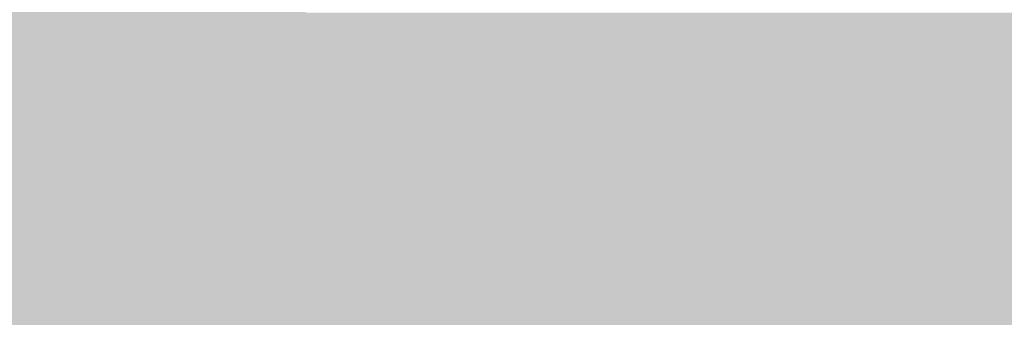
# Model space of a CAD drawing. Units: feet. Extents: x 3168 to 4724, y 827 to 1477.
# Tile 124 of 256: x 3298.685 to 3300.858, y 1098.344 to 1099.001. Entities that reach past the tile are written whole.
import ezdxf

# ---------------------------------------------------------------- set-up
doc = ezdxf.new("R2010")
doc.units = ezdxf.units.FT
doc.layers.add('A-ELEV', color=7, linetype='Continuous', lineweight=35)
doc.layers.add('A-ELEV-PATT', color=8, linetype='Continuous', lineweight=13)

msp = doc.modelspace()

# ---------------------------------------------------------------- hatches: boundary and pattern name
at = {"layer": 'A-ELEV-PATT'}
h = msp.add_hatch(color=256, dxfattribs=at)
h.dxf.hatch_style = 1
edge = h.paths.add_edge_path()
edge.add_ellipse((3552.9058, 979.2201), major_axis=(36.7449, 0), ratio=0.4848485, start_angle=0, end_angle=360)
edge = h.paths.add_edge_path()
edge.add_ellipse((3559.8916, 929.2523), major_axis=(36.7449, 0), ratio=0.4848485, start_angle=0, end_angle=360)
edge = h.paths.add_edge_path()
edge.add_line((3299.3168, 1198.6061), (3479.9167, 1198.6061))
edge.add_line((3479.9167, 1198.6061), (3479.9167, 1209.8686))
edge.add_spline(control_points=[(3479.9167, 1209.8686), (3464.3012, 1209.8686), (3448.6856, 1209.8686), (3410.9491, 1209.8686), (3388.8282, 1209.8686), (3355.6469, 1209.8686), (3344.5864, 1209.8686), (3327.9957, 1209.8686), (3322.4655, 1209.8686), (3314.1702, 1209.8686), (3311.4051, 1209.8686), (3307.2574, 1209.8686), (3305.8748, 1209.8686), (3303.801, 1209.8686), (3303.1097, 1209.8686), (3302.0728, 1209.8686), (3301.7272, 1209.8686), (3301.2087, 1209.8686), (3301.0359, 1209.8686), (3300.7767, 1209.8686), (3300.6903, 1209.8686), (3300.5606, 1209.8686), (3300.5174, 1209.8686), (3300.4526, 1209.8686), (3300.431, 1209.8686), (3300.3986, 1209.8686), (3300.3878, 1209.8686), (3300.3662, 1209.8686), (3300.3457, 1209.8686), (3300.3455, 1209.8686), (3300.3455, 1209.8686), (3300.3433, 1209.8686), (3300.3411, 1209.8686), (3300.3379, 1209.8686), (3300.3368, 1209.8686), (3300.3339, 1209.8686), (3300.3321, 1209.8686), (3300.3255, 1209.8686), (3300.3207, 1209.8686), (3300.3109, 1209.8686), (3300.306, 1209.8686), (3300.2905, 1209.8686), (3300.28, 1209.8686), (3300.2324, 1209.8688), (3300.1953, 1209.869), (3299.9511, 1209.8706), (3299.7448, 1209.8743), (3299.4368, 1209.8833), (3299.3344, 1209.8868), (3299.1811, 1209.8929), (3299.13, 1209.8951), (3298.6522, 1209.9168), (3298.2295, 1209.9457), (3297.6016, 1210.0024), (3297.3934, 1210.0235), (3297.0827, 1210.0583), (3296.9793, 1210.0705), (3296.293, 1210.1549), (3295.7181, 1210.2434), (3294.8687, 1210.3989), (3294.5877, 1210.4545), (3294.1693, 1210.5433), (3294.0304, 1210.5739), (3291.7071, 1211.1012), (3289.6536, 1211.8134), (3285.7763, 1213.564), (3283.9514, 1214.6035), (3280.5122, 1216.9801), (3278.8972, 1218.3176), (3276.3799, 1220.8295), (3275.416, 1221.9177), (3274.0393, 1223.7077), (3273.581, 1224.3495), (3273.1432, 1225.0163)], knot_values=[39.119033, 39.119033, 39.119033, 39.119033, 39.286353, 39.286353, 39.523379, 39.523379, 39.641892, 39.641892, 39.701148, 39.701148, 39.730777, 39.730777, 39.745591, 39.745591, 39.752998, 39.752998, 39.756701, 39.756701, 39.758553, 39.758553, 39.759479, 39.759479, 39.759942, 39.759942, 39.760173, 39.760173, 39.760289, 39.760289, 39.760405, 39.760405, 39.760463, 39.760463, 39.763389, 39.763389, 39.764851, 39.764851, 39.767304, 39.767304, 39.773825, 39.773825, 39.78057, 39.78057, 39.79477, 39.79477, 39.845194, 39.845194, 40.126715, 40.126715, 40.267476, 40.267476, 40.337856, 40.337856, 40.927023, 40.927023, 41.221606, 41.221606, 41.368898, 41.368898, 42.202622, 42.202622, 42.619485, 42.619485, 42.827916, 42.827916, 46.118323, 46.118323, 49.408731, 49.408731, 52.699139, 52.699139, 54.927489, 54.927489, 56.104228, 56.104228, 56.104228, 56.104228], weights=[1, 1, 1, 1, 1, 1, 1, 1, 1, 1, 1, 1, 1, 1, 1, 1, 1, 1, 1, 1, 1, 1, 1, 1, 1, 1, 1, 1, 1, 1, 1, 1, 1, 1, 1, 1, 1, 1, 1, 1, 1, 1, 1, 1, 1, 1, 1, 1, 1, 1, 1, 1, 1, 1, 1, 1, 1, 1, 1, 1, 1, 1, 1, 1, 1, 1, 1, 1, 1, 1, 1, 1, 1, 1], degree=3, periodic=0)
edge.add_line((3273.1432, 1225.0163), (3273.1432, 1099.0163))
edge.add_line((3273.1432, 1099.0163), (3299.3168, 1099.0163))
edge.add_line((3299.3168, 1099.0163), (3299.3168, 1198.6061))
edge = h.paths.add_edge_path()
edge.add_line((3304.7584, 1324.1581), (3479.9167, 1324.1581))
edge.add_line((3479.9167, 1324.1581), (3479.9167, 1335.7146))
edge.add_line((3479.9167, 1335.7146), (3269.1616, 1335.7146))
edge.add_spline(control_points=[(3269.1616, 1335.7146), (3264.0242, 1335.7146), (3258.3641, 1328.9582), (3259.2643, 1323.9003)], knot_values=[0, 0, 0, 0, 15.412191, 15.412191, 15.412191, 15.412191], degree=3, periodic=0)
edge.add_line((3259.2643, 1323.9003), (3265.5168, 1288.7691))
edge.add_line((3265.5168, 1288.7691), (3275.2651, 1261.5456))
edge.add_line((3275.2651, 1261.5456), (3304.7584, 1261.5456))
edge.add_line((3304.7584, 1261.5456), (3304.7584, 1324.1581))
h = msp.add_hatch(color=256, dxfattribs=at)
h.dxf.hatch_style = 1
h.paths.add_polyline_path([(3384.5252, 1099.0163), (3335.0292, 1099.0163), (3299.3168, 1099.0163), (3273.1432, 1099.0163), (3217.5654, 1099.0163), (3168.0693, 827.1163), (3335.0292, 827.1163)])

# ---------------------------------------------------------------- linework, layer by layer
at = {"layer": 'A-ELEV'}
msp.add_open_spline([(3808.5202, 1099.0163), (3808.5202, 1141.4132), (3808.5202, 1183.8102), (3808.5202, 1226.6353), (3808.5202, 1227.0636), (3808.5202, 1227.4918), (3811.4919, 1248.9947), (3814.4635, 1270.4975), (3817.4652, 1292.2176), (3817.4952, 1292.4348), (3817.5253, 1292.652), (3817.5728, 1310.1067), (3817.6203, 1327.5615), (3817.6679, 1345.0163), (3817.6679, 1345.458), (3817.6679, 1345.8996), (3817.6679, 1346.456), (3817.6679, 1346.5708), (3817.6679, 1346.7529), (3817.6679, 1346.8201), (3817.6679, 1346.9349), (3817.6679, 1346.9823), (3817.6679, 1347.0386), (3817.6679, 1347.0474), (3817.6679, 1347.0737), (3817.6679, 1347.0593), (3817.6679, 1347.0615), (3817.6679, 1347.0627), (3817.6679, 1347.066), (3817.6679, 1347.0683), (3817.6679, 1347.075), (3817.6679, 1347.0795), (3817.6678, 1347.0929), (3817.6678, 1347.1019), (3817.6678, 1347.1288), (3817.6677, 1347.1467), (3817.6674, 1347.2004), (3817.6672, 1347.2362), (3817.6661, 1347.3434), (3817.665, 1347.4147), (3817.6608, 1347.6281), (3817.6566, 1347.7697), (3817.64, 1348.1925), (3817.6235, 1348.4716), (3817.5591, 1349.3001), (3817.4961, 1349.8406), (3817.2554, 1351.4242), (3817.0263, 1352.4288), (3816.3069, 1354.8889), (3815.7437, 1356.2687), (3814.464, 1358.8192), (3813.7464, 1359.991), (3812.1958, 1362.1723), (3811.3622, 1363.1821), (3809.5888, 1365.069), (3808.6488, 1365.9461), (3806.6543, 1367.5796), (3805.5997, 1368.3362), (3803.3529, 1369.7223), (3802.1605, 1370.3524), (3799.6008, 1371.4536), (3798.2327, 1371.9255), (3795.2801, 1372.6346), (3793.6931, 1372.8721), (3791.8694, 1372.9265), (3791.7409, 1372.9292), (3791.3534, 1372.9341), (3791.0927, 1372.9329), (3790.3041, 1372.9151), (3789.7695, 1372.8842), (3789.2092, 1372.8302), (3789.1906, 1372.8284), (3789.1349, 1372.8229), (3789.0977, 1372.8191), (3789.0484, 1372.814), (3789.0364, 1372.8127), (3789.0003, 1372.8089), (3788.9761, 1372.8063), (3788.9494, 1372.8034), (3788.9468, 1372.8031), (3788.9426, 1372.8027), (3788.941, 1372.8025), (3788.9386, 1372.8022), (3788.9378, 1372.8021), (3788.9354, 1372.8019), (3788.8675, 1372.7944), (3788.7569, 1372.7822), (3788.7015, 1372.7761), (3788.5355, 1372.7579), (3788.4249, 1372.7457), (3788.0929, 1372.7092), (3787.8715, 1372.6848), (3787.2075, 1372.6118), (3786.7648, 1372.5631), (3785.4368, 1372.417), (3784.5515, 1372.3196), (3781.8954, 1372.0274), (3780.1247, 1371.8327), (3774.8126, 1371.2483), (3771.2713, 1370.8587), (3760.6471, 1369.69), (3753.5643, 1368.9109), (3732.316, 1366.5735), (3718.1504, 1365.0152), (3694.0068, 1362.3593), (3684.0287, 1361.2617), (3674.0506, 1360.1641), (3664.6007, 1360.1641), (3655.1508, 1360.1641), (3626.8011, 1360.1641), (3607.9013, 1360.1641), (3551.2019, 1360.1641), (3513.4023, 1360.1641), (3467.7252, 1360.1641), (3459.8476, 1360.1641), (3436.2149, 1360.1641), (3420.4597, 1360.1641), (3373.1943, 1360.1641), (3341.6839, 1360.1641), (3302.8482, 1360.1641), (3295.5227, 1360.1641), (3286.0383, 1360.1641), (3283.8794, 1360.1641), (3277.4026, 1360.1641), (3273.0848, 1360.1641), (3267.7329, 1360.1641), (3266.6988, 1360.1641), (3263.5965, 1360.1641), (3261.5284, 1360.1641), (3259.2369, 1360.1641), (3259.0137, 1360.1641), (3258.344, 1360.1641), (3257.8975, 1360.1641), (3257.431, 1360.1641), (3257.411, 1360.1641), (3257.3706, 1360.1641), (3257.3755, 1360.1641), (3257.3746, 1360.1641), (3257.3739, 1360.1641), (3257.372, 1360.1641), (3257.3706, 1360.1641), (3257.3667, 1360.1641), (3257.364, 1360.1641), (3257.3561, 1360.1641), (3257.3508, 1360.164), (3257.335, 1360.164), (3257.3244, 1360.164), (3257.2928, 1360.1639), (3257.2717, 1360.1638), (3257.2084, 1360.1634), (3257.1663, 1360.163), (3257.0402, 1360.1614), (3256.9563, 1360.1598), (3256.7055, 1360.1534), (3256.5392, 1360.147), (3256.0436, 1360.1219), (3255.7173, 1360.0971), (3254.7524, 1360.0005), (3254.128, 1359.9065), (3252.1801, 1359.5253), (3250.9416, 1359.144), (3248.6702, 1358.2433), (3247.6357, 1357.7238), (3245.7326, 1356.6035), (3244.8634, 1356.0021), (3243.2531, 1354.7429), (3242.512, 1354.0847), (3240.7511, 1352.3448), (3239.801, 1351.2296), (3238.0878, 1348.8724), (3237.3247, 1347.6304), (3235.9825, 1344.9716), (3235.4022, 1343.5549), (3234.5911, 1340.8155), (3234.3109, 1339.5435), (3233.9765, 1336.8026), (3233.9221, 1335.3309), (3234.1489, 1332.5913), (3234.3495, 1331.3672), (3234.7199, 1329.9994), (3234.7524, 1329.8834), (3234.8536, 1329.5348), (3234.9259, 1329.3017), (3235.0248, 1329.0026), (3235.0469, 1328.9369), (3235.0776, 1328.8472), (3235.0859, 1328.8232), (3235.1109, 1328.7511), (3235.1278, 1328.703), (3235.148, 1328.6462), (3235.1511, 1328.6376), (3235.1561, 1328.6235), (3235.1581, 1328.618), (3235.1602, 1328.612), (3235.1656, 1328.5969), (3235.1801, 1328.5565), (3235.1903, 1328.5281), (3235.2208, 1328.4429), (3235.2411, 1328.3862), (3235.3021, 1328.2159), (3235.3427, 1328.1023), (3235.4647, 1327.7617), (3235.546, 1327.5346), (3235.79, 1326.8534), (3235.9526, 1326.3992), (3236.4405, 1325.0367), (3236.7657, 1324.1284), (3237.7415, 1321.4034), (3238.392, 1319.5868), (3240.3435, 1314.1369), (3241.6445, 1310.5036), (3245.5476, 1299.6037), (3248.1496, 1292.3371), (3255.9557, 1270.5374), (3261.1598, 1256.0042), (3267.3876, 1238.612), (3268.4114, 1235.7529), (3269.5104, 1232.6839), (3269.5856, 1232.4739), (3269.7066, 1232.1359), (3269.7524, 1232.0079), (3269.8273, 1231.7987), (3269.8564, 1231.7176), (3269.9063, 1231.5781), (3269.9272, 1231.5198), (3269.9725, 1231.3934), (3269.9968, 1231.3254), (3270.0265, 1231.2425), (3270.0318, 1231.2277), (3270.0403, 1231.204), (3270.0392, 1231.207), (3270.0394, 1231.2066), (3270.0394, 1231.2064), (3270.0396, 1231.2058), (3270.0398, 1231.2055), (3270.0402, 1231.2043), (3270.0404, 1231.2036), (3270.0413, 1231.2013), (3270.0418, 1231.1998), (3270.0434, 1231.1953), (3270.0445, 1231.1922), (3270.0478, 1231.1832), (3270.0499, 1231.1771), (3270.0564, 1231.159), (3270.0608, 1231.147), (3270.0739, 1231.1108), (3270.0826, 1231.0867), (3270.1089, 1231.0144), (3270.1266, 1230.9663), (3270.1799, 1230.8225), (3270.2159, 1230.7269), (3270.3253, 1230.4415), (3270.4, 1230.2528), (3270.6292, 1229.6914), (3270.7889, 1229.3235), (3271.2865, 1228.2383), (3271.6431, 1227.5398), (3272.7759, 1225.5153), (3273.6142, 1224.2605), (3275.416, 1221.9177), (3276.3799, 1220.8295), (3278.8972, 1218.3176), (3280.5122, 1216.9801), (3283.9514, 1214.6035), (3285.7763, 1213.564), (3289.6536, 1211.8134), (3291.7071, 1211.1012), (3294.0304, 1210.5739), (3294.1693, 1210.5433), (3294.5877, 1210.4545), (3294.8687, 1210.3989), (3295.7181, 1210.2434), (3296.293, 1210.1549), (3296.9793, 1210.0705), (3297.0827, 1210.0583), (3297.3934, 1210.0235), (3297.6016, 1210.0024), (3298.2295, 1209.9457), (3298.6522, 1209.9168), (3299.13, 1209.8951), (3299.1811, 1209.8929), (3299.3344, 1209.8868), (3299.4368, 1209.8833), (3299.7448, 1209.8743), (3299.9511, 1209.8706), (3300.1953, 1209.869), (3300.2324, 1209.8688), (3300.28, 1209.8686), (3300.2905, 1209.8686), (3300.306, 1209.8686), (3300.3109, 1209.8686), (3300.3207, 1209.8686), (3300.3255, 1209.8686), (3300.3321, 1209.8686), (3300.3339, 1209.8686), (3300.3368, 1209.8686), (3300.3379, 1209.8686), (3300.3411, 1209.8686), (3300.3433, 1209.8686), (3300.3455, 1209.8686), (3300.3455, 1209.8686), (3300.3457, 1209.8686), (3300.3662, 1209.8686), (3300.3878, 1209.8686), (3300.3986, 1209.8686), (3300.431, 1209.8686), (3300.4526, 1209.8686), (3300.5174, 1209.8686), (3300.5606, 1209.8686), (3300.6903, 1209.8686), (3300.7767, 1209.8686), (3301.0359, 1209.8686), (3301.2087, 1209.8686), (3301.7272, 1209.8686), (3302.0728, 1209.8686), (3303.1097, 1209.8686), (3303.801, 1209.8686), (3305.8748, 1209.8686), (3307.2574, 1209.8686), (3311.4051, 1209.8686), (3314.1702, 1209.8686), (3322.4655, 1209.8686), (3327.9957, 1209.8686), (3344.5864, 1209.8686), (3355.6469, 1209.8686), (3388.8282, 1209.8686), (3410.9491, 1209.8686), (3477.3119, 1209.8686), (3521.5537, 1209.8686), (3566.8362, 1209.8686), (3567.8769, 1209.8686), (3570.999, 1209.8686), (3573.0804, 1209.8686), (3575.7814, 1209.8686), (3576.4009, 1209.8686), (3577.2958, 1209.8686), (3577.5712, 1209.8686), (3578.3971, 1209.8686), (3578.9478, 1209.8686), (3579.7565, 1209.8686), (3580.0145, 1209.8686), (3580.3427, 1209.8686), (3580.3269, 1209.8686), (3580.3272, 1209.8686), (3580.3273, 1209.8686), (3580.3278, 1209.8686), (3580.3281, 1209.8686), (3580.329, 1209.8686), (3580.3296, 1209.8686), (3580.3314, 1209.8686), (3580.3327, 1209.8686), (3580.3363, 1209.8686), (3580.3388, 1209.8686), (3580.3461, 1209.8686), (3580.351, 1209.8686), (3580.3657, 1209.8685), (3580.3754, 1209.8685), (3580.4048, 1209.8684), (3580.4244, 1209.8684), (3580.4832, 1209.8681), (3580.5224, 1209.8678), (3580.6404, 1209.8666), (3580.7192, 1209.8655), (3580.9563, 1209.8608), (3581.1152, 1209.8561), (3581.5942, 1209.8372), (3581.9164, 1209.8183), (3582.8899, 1209.7424), (3583.548, 1209.6662), (3585.5318, 1209.3606), (3586.8672, 1209.0539), (3589.4715, 1208.2525), (3590.7402, 1207.7579), (3591.9955, 1207.1588), (3592.0578, 1207.1287), (3592.2442, 1207.038), (3592.3677, 1206.9766), (3592.7353, 1206.7904), (3592.9768, 1206.6631), (3593.2445, 1206.5164), (3593.2747, 1206.4998), (3593.3651, 1206.4498), (3593.4251, 1206.4163), (3593.6043, 1206.3153), (3593.7227, 1206.2472), (3593.8572, 1206.1684), (3593.8744, 1206.1583), (3593.9257, 1206.128), (3593.9599, 1206.1078), (3594.0621, 1206.0469), (3594.1298, 1206.0061), (3594.2084, 1205.9582), (3594.2197, 1205.9513), (3594.2534, 1205.9307), (3594.2758, 1205.9169), (3594.343, 1205.8755), (3594.3876, 1205.8479), (3594.4336, 1205.819), (3594.4353, 1205.818), (3594.4402, 1205.8149), (3594.4435, 1205.8129), (3594.4471, 1205.8106), (3594.4475, 1205.8103), (3594.4487, 1205.8096), (3594.4495, 1205.8091), (3594.4504, 1205.8086), (3594.4505, 1205.8085), (3594.4506, 1205.8084), (3594.4674, 1205.7979), (3594.4933, 1205.7817), (3594.5062, 1205.7736), (3594.545, 1205.7492), (3594.5709, 1205.733), (3594.6485, 1205.6844), (3594.7002, 1205.652), (3594.8554, 1205.5547), (3594.9589, 1205.4898), (3595.2694, 1205.2953), (3595.4763, 1205.1656), (3596.0972, 1204.7765), (3596.5111, 1204.5171), (3597.7528, 1203.7388), (3598.5807, 1203.22), (3601.0642, 1201.6636), (3602.7198, 1200.6259), (3607.6868, 1197.513), (3610.9981, 1195.4377), (3620.932, 1189.2119), (3627.5546, 1185.0614), (3647.4225, 1172.6097), (3660.6678, 1164.3086), (3700.4035, 1139.4053), (3726.894, 1122.8031), (3757.2057, 1103.8061), (3761.027, 1101.4112), (3764.8482, 1099.0163), (3745.3283, 1099.0163), (3725.8083, 1099.0163), (3706.2884, 1099.0163), (3706.2884, 1108.4532), (3706.2884, 1117.8902), (3706.2884, 1127.3271), (3710.7508, 1127.3271), (3715.2131, 1127.3271), (3719.6755, 1127.3271)], degree=3, knots=[0, 0, 0, 0, 0.982037, 0.982037, 0.991957, 0.991957, 0.991957, 1.966522, 1.966522, 1.976367, 1.976367, 1.976367, 2.976367, 2.976367, 2.976367, 3.00169, 3.00169, 3.008272, 3.008272, 3.012129, 3.012129, 3.014851, 3.014851, 3.015353, 3.015353, 3.016359, 3.016359, 3.017365, 3.017365, 3.019376, 3.019376, 3.023398, 3.023398, 3.031442, 3.031442, 3.047531, 3.047531, 3.079708, 3.079708, 3.144063, 3.144063, 3.272772, 3.272772, 3.53019, 3.53019, 4.045026, 4.045026, 5.074698, 5.074698, 6.700878, 6.700878, 8.327058, 8.327058, 9.953238, 9.953238, 11.579418, 11.579418, 13.205598, 13.205598, 14.831778, 14.831778, 16.457958, 16.457958, 18.084138, 18.084138, 18.206872, 18.206872, 18.45234, 18.45234, 18.943275, 18.943275, 18.960093, 18.960093, 18.993729, 18.993729, 19.00461, 19.00461, 19.026374, 19.026374, 19.028737, 19.028737, 19.03018, 19.03018, 19.030897, 19.030897, 19.032332, 19.032332, 19.033766, 19.033766, 19.036636, 19.036636, 19.042374, 19.042374, 19.053851, 19.053851, 19.076805, 19.076805, 19.122714, 19.122714, 19.21453, 19.21453, 19.398163, 19.398163, 19.765429, 19.765429, 20.024128, 20.024128, 20.024128, 20.092031, 20.092031, 20.227836, 20.227836, 20.499446, 20.499446, 20.556051, 20.556051, 20.66926, 20.66926, 20.895678, 20.895678, 20.948316, 20.948316, 20.963829, 20.963829, 20.994855, 20.994855, 21.002285, 21.002285, 21.017146, 21.017146, 21.01875, 21.01875, 21.021959, 21.021959, 21.022102, 21.022102, 21.022249, 21.022249, 21.022708, 21.022708, 21.023627, 21.023627, 21.025464, 21.025464, 21.029138, 21.029138, 21.036486, 21.036486, 21.051183, 21.051183, 21.080575, 21.080575, 21.139361, 21.139361, 21.256932, 21.256932, 21.492073, 21.492073, 21.962356, 21.962356, 23.01002, 23.01002, 24.057684, 24.057684, 25.105348, 25.105348, 26.153011, 26.153011, 27.776787, 27.776787, 29.400562, 29.400562, 31.024337, 31.024337, 32.278801, 32.278801, 33.533265, 33.533265, 34.467568, 34.467568, 34.553971, 34.553971, 34.726776, 34.726776, 34.775309, 34.775309, 34.793079, 34.793079, 34.82862, 34.82862, 34.834979, 34.834979, 34.839039, 34.839039, 34.839411, 34.839411, 34.840285, 34.840285, 34.842034, 34.842034, 34.845531, 34.845531, 34.852525, 34.852525, 34.866512, 34.866512, 34.894488, 34.894488, 34.950439, 34.950439, 35.062342, 35.062342, 35.286147, 35.286147, 35.733758, 35.733758, 35.821815, 35.821815, 35.828283, 35.828283, 35.832225, 35.832225, 35.834724, 35.834724, 35.836521, 35.836521, 35.838617, 35.838617, 35.839073, 35.839073, 35.839345, 35.839345, 35.839617, 35.839617, 35.840161, 35.840161, 35.841249, 35.841249, 35.843425, 35.843425, 35.847778, 35.847778, 35.856482, 35.856482, 35.873891, 35.873891, 35.908709, 35.908709, 35.978345, 35.978345, 36.117617, 36.117617, 36.396161, 36.396161, 36.953248, 36.953248, 38.067423, 38.067423, 40.295772, 40.295772, 42.524122, 42.524122, 45.81453, 45.81453, 49.104937, 49.104937, 52.395345, 52.395345, 52.603776, 52.603776, 53.020639, 53.020639, 53.854363, 53.854363, 54.001655, 54.001655, 54.296238, 54.296238, 54.885405, 54.885405, 54.955785, 54.955785, 55.096546, 55.096546, 55.378067, 55.378067, 55.42849, 55.42849, 55.442691, 55.442691, 55.449436, 55.449436, 55.455957, 55.455957, 55.458409, 55.458409, 55.459872, 55.459872, 55.462798, 55.462798, 55.462856, 55.462856, 55.462972, 55.462972, 55.463088, 55.463088, 55.463319, 55.463319, 55.463782, 55.463782, 55.464708, 55.464708, 55.46656, 55.46656, 55.470263, 55.470263, 55.47767, 55.47767, 55.492484, 55.492484, 55.522112, 55.522112, 55.581369, 55.581369, 55.699882, 55.699882, 55.936907, 55.936907, 56.410959, 56.410959, 56.42211, 56.42211, 56.444413, 56.444413, 56.451051, 56.451051, 56.454001, 56.454001, 56.459901, 56.459901, 56.462666, 56.462666, 56.463418, 56.463418, 56.464171, 56.464171, 56.465675, 56.465675, 56.468684, 56.468684, 56.474702, 56.474702, 56.486738, 56.486738, 56.51081, 56.51081, 56.558955, 56.558955, 56.655243, 56.655243, 56.847821, 56.847821, 57.232975, 57.232975, 58.003284, 58.003284, 59.543901, 59.543901, 62.625137, 62.625137, 68.787607, 68.787607, 74.950078, 74.950078, 75.27336, 75.27336, 75.919923, 75.919923, 77.213051, 77.213051, 77.377769, 77.377769, 77.707206, 77.707206, 78.366079, 78.366079, 78.462532, 78.462532, 78.655436, 78.655436, 79.041245, 79.041245, 79.105735, 79.105735, 79.234714, 79.234714, 79.492672, 79.492672, 79.502197, 79.502197, 79.521249, 79.521249, 79.523534, 79.523534, 79.528103, 79.528103, 79.528682, 79.528682, 79.528885, 79.528885, 79.529089, 79.529089, 79.529495, 79.529495, 79.530308, 79.530308, 79.531935, 79.531935, 79.535187, 79.535187, 79.541693, 79.541693, 79.554704, 79.554704, 79.580725, 79.580725, 79.632769, 79.632769, 79.736856, 79.736856, 79.94503, 79.94503, 80.361377, 80.361377, 80.421435, 80.421435, 80.421435, 81.421435, 81.421435, 81.421435, 82.421435, 82.421435, 82.421435, 83.421435, 83.421435, 83.421435, 83.421435], dxfattribs=at)

doc.saveas('drawing.dxf')
